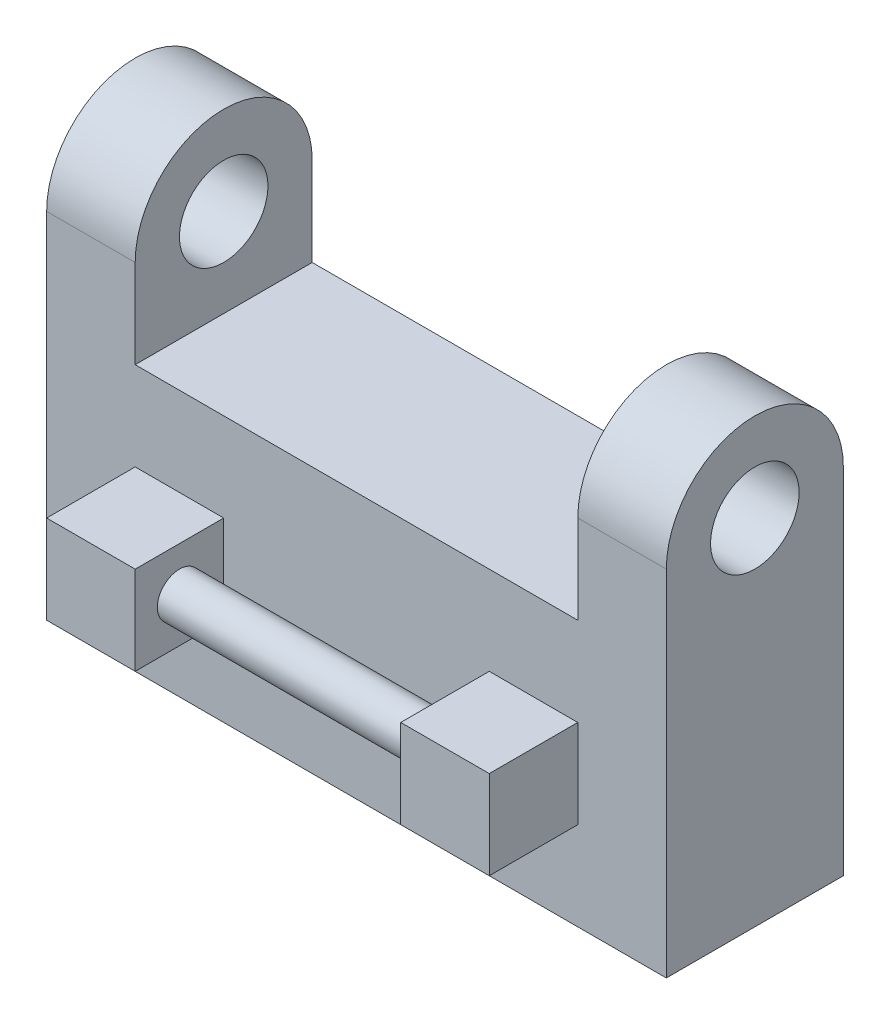
ISO-10303-21;
HEADER;
FILE_DESCRIPTION(('STEP AP214'),'2;1');
FILE_NAME('part.step','',(''),(''),'','','');
FILE_SCHEMA(('AUTOMOTIVE_DESIGN { 1 0 10303 214 1 1 1 1 }'));
ENDSEC;
DATA;
#1=APPLICATION_CONTEXT('core data for automotive mechanical design processes');
#2=APPLICATION_PROTOCOL_DEFINITION('international standard','automotive_design',2000,#1);
#3=PRODUCT_CONTEXT('',#1,'mechanical');
#4=PRODUCT('Part','Part','',(#3));
#5=PRODUCT_RELATED_PRODUCT_CATEGORY('part','',(#4));
#6=PRODUCT_DEFINITION_FORMATION('','',#4);
#7=PRODUCT_DEFINITION_CONTEXT('part definition',#1,'design');
#8=PRODUCT_DEFINITION('design','',#6,#7);
#9=PRODUCT_DEFINITION_SHAPE('','',#8);
#10=(LENGTH_UNIT() NAMED_UNIT(*) SI_UNIT(.MILLI.,.METRE.));
#11=(NAMED_UNIT(*) PLANE_ANGLE_UNIT() SI_UNIT($,.RADIAN.));
#12=(NAMED_UNIT(*) SI_UNIT($,.STERADIAN.) SOLID_ANGLE_UNIT());
#13=UNCERTAINTY_MEASURE_WITH_UNIT(LENGTH_MEASURE(1.E-05),#10,'distance_accuracy_value','');
#14=(GEOMETRIC_REPRESENTATION_CONTEXT(3) GLOBAL_UNCERTAINTY_ASSIGNED_CONTEXT((#13)) GLOBAL_UNIT_ASSIGNED_CONTEXT((#10,
#11,#12)) REPRESENTATION_CONTEXT('',''));
#15=CARTESIAN_POINT('',(0.,0.,0.));
#16=DIRECTION('',(0.,0.,1.));
#17=DIRECTION('',(1.,0.,0.));
#18=AXIS2_PLACEMENT_3D('',#15,#16,#17);
#19=CARTESIAN_POINT('',(0.,0.,20.));
#20=DIRECTION('',(0.,0.,1.));
#21=DIRECTION('',(1.,0.,0.));
#22=AXIS2_PLACEMENT_3D('',#19,#20,#21);
#23=PLANE('',#22);
#24=DIRECTION('',(0.,-1.,0.));
#25=VECTOR('',#24,1.);
#26=CARTESIAN_POINT('',(0.,30.,20.));
#27=LINE('',#26,#25);
#28=CARTESIAN_POINT('',(0.,40.,20.));
#29=VERTEX_POINT('',#28);
#30=CARTESIAN_POINT('',(0.,0.,20.));
#31=VERTEX_POINT('',#30);
#32=EDGE_CURVE('E389',#29,#31,#27,.T.);
#33=ORIENTED_EDGE('',*,*,#32,.T.);
#34=DIRECTION('',(1.,0.,0.));
#35=VECTOR('',#34,1.);
#36=CARTESIAN_POINT('',(0.,0.,20.));
#37=LINE('',#36,#35);
#38=CARTESIAN_POINT('',(70.,0.,20.));
#39=VERTEX_POINT('',#38);
#40=EDGE_CURVE('E392',#31,#39,#37,.T.);
#41=ORIENTED_EDGE('',*,*,#40,.T.);
#42=DIRECTION('',(0.,1.,0.));
#43=VECTOR('',#42,1.);
#44=CARTESIAN_POINT('',(70.,0.,20.));
#45=LINE('',#44,#43);
#46=CARTESIAN_POINT('',(70.,40.,20.));
#47=VERTEX_POINT('',#46);
#48=EDGE_CURVE('E391',#39,#47,#45,.T.);
#49=ORIENTED_EDGE('',*,*,#48,.T.);
#50=DIRECTION('',(1.,0.,0.));
#51=VECTOR('',#50,1.);
#52=CARTESIAN_POINT('',(60.,40.,20.));
#53=LINE('',#52,#51);
#54=CARTESIAN_POINT('',(60.,40.,20.));
#55=VERTEX_POINT('',#54);
#56=EDGE_CURVE('E351',#55,#47,#53,.T.);
#57=ORIENTED_EDGE('',*,*,#56,.F.);
#58=DIRECTION('',(0.,-1.,0.));
#59=VECTOR('',#58,1.);
#60=CARTESIAN_POINT('',(60.,40.,20.));
#61=LINE('',#60,#59);
#62=CARTESIAN_POINT('',(60.,30.,20.));
#63=VERTEX_POINT('',#62);
#64=EDGE_CURVE('E348',#55,#63,#61,.T.);
#65=ORIENTED_EDGE('',*,*,#64,.T.);
#66=DIRECTION('',(-1.,0.,0.));
#67=VECTOR('',#66,1.);
#68=CARTESIAN_POINT('',(70.,30.,20.));
#69=LINE('',#68,#67);
#70=CARTESIAN_POINT('',(10.,30.,20.));
#71=VERTEX_POINT('',#70);
#72=EDGE_CURVE('E398',#63,#71,#69,.T.);
#73=ORIENTED_EDGE('',*,*,#72,.T.);
#74=DIRECTION('',(0.,-1.,0.));
#75=VECTOR('',#74,1.);
#76=CARTESIAN_POINT('',(10.,40.,20.));
#77=LINE('',#76,#75);
#78=CARTESIAN_POINT('',(10.,40.,20.));
#79=VERTEX_POINT('',#78);
#80=EDGE_CURVE('E371',#79,#71,#77,.T.);
#81=ORIENTED_EDGE('',*,*,#80,.F.);
#82=DIRECTION('',(-1.,0.,0.));
#83=VECTOR('',#82,1.);
#84=CARTESIAN_POINT('',(10.,40.,20.));
#85=LINE('',#84,#83);
#86=EDGE_CURVE('E381',#79,#29,#85,.T.);
#87=ORIENTED_EDGE('',*,*,#86,.T.);
#88=EDGE_LOOP('',(#33,#41,#49,#57,#65,#73,#81,#87));
#89=FACE_BOUND('',#88,.T.);
#90=DIRECTION('',(-1.,0.,0.));
#91=VECTOR('',#90,1.);
#92=CARTESIAN_POINT('',(50.,20.,20.));
#93=LINE('',#92,#91);
#94=CARTESIAN_POINT('',(60.,20.,20.));
#95=VERTEX_POINT('',#94);
#96=CARTESIAN_POINT('',(50.,20.,20.));
#97=VERTEX_POINT('',#96);
#98=EDGE_CURVE('E316',#95,#97,#93,.T.);
#99=ORIENTED_EDGE('',*,*,#98,.F.);
#100=DIRECTION('',(0.,1.,0.));
#101=VECTOR('',#100,1.);
#102=CARTESIAN_POINT('',(60.,20.,20.));
#103=LINE('',#102,#101);
#104=CARTESIAN_POINT('',(60.,10.,20.));
#105=VERTEX_POINT('',#104);
#106=EDGE_CURVE('E304',#105,#95,#103,.T.);
#107=ORIENTED_EDGE('',*,*,#106,.F.);
#108=DIRECTION('',(1.,0.,0.));
#109=VECTOR('',#108,1.);
#110=CARTESIAN_POINT('',(50.,10.,20.));
#111=LINE('',#110,#109);
#112=CARTESIAN_POINT('',(50.,10.,20.));
#113=VERTEX_POINT('',#112);
#114=EDGE_CURVE('E309',#113,#105,#111,.T.);
#115=ORIENTED_EDGE('',*,*,#114,.F.);
#116=DIRECTION('',(0.,-1.,0.));
#117=VECTOR('',#116,1.);
#118=CARTESIAN_POINT('',(50.,20.,20.));
#119=LINE('',#118,#117);
#120=EDGE_CURVE('E322',#97,#113,#119,.T.);
#121=ORIENTED_EDGE('',*,*,#120,.F.);
#122=EDGE_LOOP('',(#99,#107,#115,#121));
#123=FACE_BOUND('',#122,.T.);
#124=DIRECTION('',(1.,0.,0.));
#125=VECTOR('',#124,1.);
#126=CARTESIAN_POINT('',(10.,10.,20.));
#127=LINE('',#126,#125);
#128=CARTESIAN_POINT('',(10.,10.,20.));
#129=VERTEX_POINT('',#128);
#130=CARTESIAN_POINT('',(20.,10.,20.));
#131=VERTEX_POINT('',#130);
#132=EDGE_CURVE('E287',#129,#131,#127,.T.);
#133=ORIENTED_EDGE('',*,*,#132,.F.);
#134=DIRECTION('',(0.,-1.,0.));
#135=VECTOR('',#134,1.);
#136=CARTESIAN_POINT('',(9.99999999999999,20.,20.));
#137=LINE('',#136,#135);
#138=CARTESIAN_POINT('',(9.99999999999999,20.,20.));
#139=VERTEX_POINT('',#138);
#140=EDGE_CURVE('E277',#139,#129,#137,.T.);
#141=ORIENTED_EDGE('',*,*,#140,.F.);
#142=DIRECTION('',(-1.,0.,0.));
#143=VECTOR('',#142,1.);
#144=CARTESIAN_POINT('',(9.99999999999999,20.,20.));
#145=LINE('',#144,#143);
#146=CARTESIAN_POINT('',(20.,20.,20.));
#147=VERTEX_POINT('',#146);
#148=EDGE_CURVE('E282',#147,#139,#145,.T.);
#149=ORIENTED_EDGE('',*,*,#148,.F.);
#150=DIRECTION('',(0.,1.,0.));
#151=VECTOR('',#150,1.);
#152=CARTESIAN_POINT('',(20.,20.,20.));
#153=LINE('',#152,#151);
#154=EDGE_CURVE('E292',#131,#147,#153,.T.);
#155=ORIENTED_EDGE('',*,*,#154,.F.);
#156=EDGE_LOOP('',(#133,#141,#149,#155));
#157=FACE_BOUND('',#156,.T.);
#158=ADVANCED_FACE('F44',(#89,#123,#157),#23,.T.);
#159=CARTESIAN_POINT('',(70.,30.,20.));
#160=DIRECTION('',(0.,-1.,0.));
#161=DIRECTION('',(0.,0.,-1.));
#162=AXIS2_PLACEMENT_3D('',#159,#160,#161);
#163=PLANE('',#162);
#164=ORIENTED_EDGE('',*,*,#72,.F.);
#165=DIRECTION('',(0.,0.,-1.));
#166=VECTOR('',#165,1.);
#167=CARTESIAN_POINT('',(60.,30.,0.));
#168=LINE('',#167,#166);
#169=CARTESIAN_POINT('',(60.,30.,0.));
#170=VERTEX_POINT('',#169);
#171=EDGE_CURVE('E350',#63,#170,#168,.T.);
#172=ORIENTED_EDGE('',*,*,#171,.T.);
#173=DIRECTION('',(-1.,0.,0.));
#174=VECTOR('',#173,1.);
#175=CARTESIAN_POINT('',(70.,30.,0.));
#176=LINE('',#175,#174);
#177=CARTESIAN_POINT('',(10.,30.,0.));
#178=VERTEX_POINT('',#177);
#179=EDGE_CURVE('E395',#170,#178,#176,.T.);
#180=ORIENTED_EDGE('',*,*,#179,.T.);
#181=DIRECTION('',(0.,0.,-1.));
#182=VECTOR('',#181,1.);
#183=CARTESIAN_POINT('',(10.,30.,0.));
#184=LINE('',#183,#182);
#185=EDGE_CURVE('E372',#71,#178,#184,.T.);
#186=ORIENTED_EDGE('',*,*,#185,.F.);
#187=EDGE_LOOP('',(#164,#172,#180,#186));
#188=FACE_BOUND('',#187,.T.);
#189=ADVANCED_FACE('F432',(#188),#163,.F.);
#190=CARTESIAN_POINT('',(0.,30.,20.));
#191=DIRECTION('',(1.,0.,0.));
#192=DIRECTION('',(0.,0.,-1.));
#193=AXIS2_PLACEMENT_3D('',#190,#191,#192);
#194=PLANE('',#193);
#195=DIRECTION('',(0.,-1.,0.));
#196=VECTOR('',#195,1.);
#197=CARTESIAN_POINT('',(0.,30.,0.));
#198=LINE('',#197,#196);
#199=CARTESIAN_POINT('',(0.,40.,0.));
#200=VERTEX_POINT('',#199);
#201=CARTESIAN_POINT('',(0.,0.,0.));
#202=VERTEX_POINT('',#201);
#203=EDGE_CURVE('E390',#200,#202,#198,.T.);
#204=ORIENTED_EDGE('',*,*,#203,.T.);
#205=DIRECTION('',(0.,0.,-1.));
#206=VECTOR('',#205,1.);
#207=CARTESIAN_POINT('',(0.,0.,20.));
#208=LINE('',#207,#206);
#209=EDGE_CURVE('E409',#31,#202,#208,.T.);
#210=ORIENTED_EDGE('',*,*,#209,.F.);
#211=ORIENTED_EDGE('',*,*,#32,.F.);
#212=CARTESIAN_POINT('',(0.,40.,10.));
#213=DIRECTION('',(1.,0.,0.));
#214=DIRECTION('',(0.,0.,-1.));
#215=AXIS2_PLACEMENT_3D('',#212,#213,#214);
#216=CIRCLE('',#215,10.);
#217=EDGE_CURVE('E362',#200,#29,#216,.T.);
#218=ORIENTED_EDGE('',*,*,#217,.F.);
#219=EDGE_LOOP('',(#204,#210,#211,#218));
#220=FACE_BOUND('',#219,.T.);
#221=CARTESIAN_POINT('',(0.,40.,10.));
#222=DIRECTION('',(1.,0.,0.));
#223=DIRECTION('',(0.,0.,-1.));
#224=AXIS2_PLACEMENT_3D('',#221,#222,#223);
#225=CIRCLE('',#224,5.);
#226=CARTESIAN_POINT('',(0.,40.,5.));
#227=VERTEX_POINT('',#226);
#228=EDGE_CURVE('E363',#227,#227,#225,.T.);
#229=ORIENTED_EDGE('',*,*,#228,.T.);
#230=EDGE_LOOP('',(#229));
#231=FACE_BOUND('',#230,.T.);
#232=ADVANCED_FACE('F50',(#220,#231),#194,.F.);
#233=CARTESIAN_POINT('',(0.,0.,20.));
#234=DIRECTION('',(0.,1.,0.));
#235=DIRECTION('',(0.,0.,1.));
#236=AXIS2_PLACEMENT_3D('',#233,#234,#235);
#237=PLANE('',#236);
#238=DIRECTION('',(1.,0.,0.));
#239=VECTOR('',#238,1.);
#240=CARTESIAN_POINT('',(0.,0.,0.));
#241=LINE('',#240,#239);
#242=CARTESIAN_POINT('',(70.,0.,0.));
#243=VERTEX_POINT('',#242);
#244=EDGE_CURVE('E402',#202,#243,#241,.T.);
#245=ORIENTED_EDGE('',*,*,#244,.T.);
#246=DIRECTION('',(0.,0.,-1.));
#247=VECTOR('',#246,1.);
#248=CARTESIAN_POINT('',(70.,0.,20.));
#249=LINE('',#248,#247);
#250=EDGE_CURVE('E396',#39,#243,#249,.T.);
#251=ORIENTED_EDGE('',*,*,#250,.F.);
#252=ORIENTED_EDGE('',*,*,#40,.F.);
#253=ORIENTED_EDGE('',*,*,#209,.T.);
#254=EDGE_LOOP('',(#245,#251,#252,#253));
#255=FACE_BOUND('',#254,.T.);
#256=ADVANCED_FACE('F451',(#255),#237,.F.);
#257=CARTESIAN_POINT('',(70.,0.,20.));
#258=DIRECTION('',(-1.,0.,0.));
#259=DIRECTION('',(0.,0.,1.));
#260=AXIS2_PLACEMENT_3D('',#257,#258,#259);
#261=PLANE('',#260);
#262=DIRECTION('',(0.,1.,0.));
#263=VECTOR('',#262,1.);
#264=CARTESIAN_POINT('',(70.,0.,0.));
#265=LINE('',#264,#263);
#266=CARTESIAN_POINT('',(70.,40.,0.));
#267=VERTEX_POINT('',#266);
#268=EDGE_CURVE('E401',#243,#267,#265,.T.);
#269=ORIENTED_EDGE('',*,*,#268,.T.);
#270=CARTESIAN_POINT('',(70.,40.,10.));
#271=DIRECTION('',(1.,0.,0.));
#272=DIRECTION('',(0.,0.,-1.));
#273=AXIS2_PLACEMENT_3D('',#270,#271,#272);
#274=CIRCLE('',#273,10.);
#275=EDGE_CURVE('E336',#267,#47,#274,.T.);
#276=ORIENTED_EDGE('',*,*,#275,.T.);
#277=ORIENTED_EDGE('',*,*,#48,.F.);
#278=ORIENTED_EDGE('',*,*,#250,.T.);
#279=EDGE_LOOP('',(#269,#276,#277,#278));
#280=FACE_BOUND('',#279,.T.);
#281=CARTESIAN_POINT('',(70.,40.,10.));
#282=DIRECTION('',(1.,0.,0.));
#283=DIRECTION('',(0.,0.,-1.));
#284=AXIS2_PLACEMENT_3D('',#281,#282,#283);
#285=CIRCLE('',#284,5.);
#286=CARTESIAN_POINT('',(70.,40.,5.));
#287=VERTEX_POINT('',#286);
#288=EDGE_CURVE('E334',#287,#287,#285,.T.);
#289=ORIENTED_EDGE('',*,*,#288,.F.);
#290=EDGE_LOOP('',(#289));
#291=FACE_BOUND('',#290,.T.);
#292=ADVANCED_FACE('F448',(#280,#291),#261,.F.);
#293=CARTESIAN_POINT('',(0.,0.,0.));
#294=DIRECTION('',(0.,0.,1.));
#295=DIRECTION('',(1.,0.,0.));
#296=AXIS2_PLACEMENT_3D('',#293,#294,#295);
#297=PLANE('',#296);
#298=DIRECTION('',(-1.,0.,0.));
#299=VECTOR('',#298,1.);
#300=CARTESIAN_POINT('',(9.99999999999999,20.,0.));
#301=LINE('',#300,#299);
#302=CARTESIAN_POINT('',(20.,20.,0.));
#303=VERTEX_POINT('',#302);
#304=CARTESIAN_POINT('',(9.99999999999999,20.,0.));
#305=VERTEX_POINT('',#304);
#306=EDGE_CURVE('E238',#303,#305,#301,.T.);
#307=ORIENTED_EDGE('',*,*,#306,.T.);
#308=DIRECTION('',(0.,-1.,0.));
#309=VECTOR('',#308,1.);
#310=CARTESIAN_POINT('',(9.99999999999999,20.,0.));
#311=LINE('',#310,#309);
#312=CARTESIAN_POINT('',(10.,10.,0.));
#313=VERTEX_POINT('',#312);
#314=EDGE_CURVE('E215',#305,#313,#311,.T.);
#315=ORIENTED_EDGE('',*,*,#314,.T.);
#316=DIRECTION('',(1.,0.,0.));
#317=VECTOR('',#316,1.);
#318=CARTESIAN_POINT('',(10.,10.,0.));
#319=LINE('',#318,#317);
#320=CARTESIAN_POINT('',(20.,10.,0.));
#321=VERTEX_POINT('',#320);
#322=EDGE_CURVE('E226',#313,#321,#319,.T.);
#323=ORIENTED_EDGE('',*,*,#322,.T.);
#324=DIRECTION('',(0.,1.,0.));
#325=VECTOR('',#324,1.);
#326=CARTESIAN_POINT('',(20.,20.,0.));
#327=LINE('',#326,#325);
#328=EDGE_CURVE('E58',#321,#303,#327,.T.);
#329=ORIENTED_EDGE('',*,*,#328,.T.);
#330=EDGE_LOOP('',(#307,#315,#323,#329));
#331=FACE_BOUND('',#330,.T.);
#332=DIRECTION('',(1.,0.,0.));
#333=VECTOR('',#332,1.);
#334=CARTESIAN_POINT('',(50.,10.,0.));
#335=LINE('',#334,#333);
#336=CARTESIAN_POINT('',(50.,10.,0.));
#337=VERTEX_POINT('',#336);
#338=CARTESIAN_POINT('',(60.,10.,0.));
#339=VERTEX_POINT('',#338);
#340=EDGE_CURVE('E264',#337,#339,#335,.T.);
#341=ORIENTED_EDGE('',*,*,#340,.T.);
#342=DIRECTION('',(0.,1.,0.));
#343=VECTOR('',#342,1.);
#344=CARTESIAN_POINT('',(60.,20.,0.));
#345=LINE('',#344,#343);
#346=CARTESIAN_POINT('',(60.,20.,0.));
#347=VERTEX_POINT('',#346);
#348=EDGE_CURVE('E220',#339,#347,#345,.T.);
#349=ORIENTED_EDGE('',*,*,#348,.T.);
#350=DIRECTION('',(-1.,0.,0.));
#351=VECTOR('',#350,1.);
#352=CARTESIAN_POINT('',(50.,20.,0.));
#353=LINE('',#352,#351);
#354=CARTESIAN_POINT('',(50.,20.,0.));
#355=VERTEX_POINT('',#354);
#356=EDGE_CURVE('E252',#347,#355,#353,.T.);
#357=ORIENTED_EDGE('',*,*,#356,.T.);
#358=DIRECTION('',(0.,-1.,0.));
#359=VECTOR('',#358,1.);
#360=CARTESIAN_POINT('',(50.,20.,0.));
#361=LINE('',#360,#359);
#362=EDGE_CURVE('E69',#355,#337,#361,.T.);
#363=ORIENTED_EDGE('',*,*,#362,.T.);
#364=EDGE_LOOP('',(#341,#349,#357,#363));
#365=FACE_BOUND('',#364,.T.);
#366=ORIENTED_EDGE('',*,*,#203,.F.);
#367=DIRECTION('',(-1.,0.,0.));
#368=VECTOR('',#367,1.);
#369=CARTESIAN_POINT('',(10.,40.,0.));
#370=LINE('',#369,#368);
#371=CARTESIAN_POINT('',(10.,40.,0.));
#372=VERTEX_POINT('',#371);
#373=EDGE_CURVE('E378',#372,#200,#370,.T.);
#374=ORIENTED_EDGE('',*,*,#373,.F.);
#375=DIRECTION('',(0.,1.,0.));
#376=VECTOR('',#375,1.);
#377=CARTESIAN_POINT('',(10.,40.,0.));
#378=LINE('',#377,#376);
#379=EDGE_CURVE('E380',#178,#372,#378,.T.);
#380=ORIENTED_EDGE('',*,*,#379,.F.);
#381=ORIENTED_EDGE('',*,*,#179,.F.);
#382=DIRECTION('',(0.,1.,0.));
#383=VECTOR('',#382,1.);
#384=CARTESIAN_POINT('',(60.,40.,0.));
#385=LINE('',#384,#383);
#386=CARTESIAN_POINT('',(60.,40.,0.));
#387=VERTEX_POINT('',#386);
#388=EDGE_CURVE('E341',#170,#387,#385,.T.);
#389=ORIENTED_EDGE('',*,*,#388,.T.);
#390=DIRECTION('',(1.,0.,0.));
#391=VECTOR('',#390,1.);
#392=CARTESIAN_POINT('',(60.,40.,0.));
#393=LINE('',#392,#391);
#394=EDGE_CURVE('E356',#387,#267,#393,.T.);
#395=ORIENTED_EDGE('',*,*,#394,.T.);
#396=ORIENTED_EDGE('',*,*,#268,.F.);
#397=ORIENTED_EDGE('',*,*,#244,.F.);
#398=EDGE_LOOP('',(#366,#374,#380,#381,#389,#395,#396,#397));
#399=FACE_BOUND('',#398,.T.);
#400=ADVANCED_FACE('F450',(#331,#365,#399),#297,.F.);
#401=CARTESIAN_POINT('',(10.,40.,10.));
#402=DIRECTION('',(1.,0.,0.));
#403=DIRECTION('',(0.,0.,-1.));
#404=AXIS2_PLACEMENT_3D('',#401,#402,#403);
#405=PLANE('',#404);
#406=CARTESIAN_POINT('',(10.,40.,10.));
#407=DIRECTION('',(1.,0.,0.));
#408=DIRECTION('',(0.,0.,-1.));
#409=AXIS2_PLACEMENT_3D('',#406,#407,#408);
#410=CIRCLE('',#409,10.);
#411=EDGE_CURVE('E368',#372,#79,#410,.T.);
#412=ORIENTED_EDGE('',*,*,#411,.T.);
#413=ORIENTED_EDGE('',*,*,#80,.T.);
#414=ORIENTED_EDGE('',*,*,#185,.T.);
#415=ORIENTED_EDGE('',*,*,#379,.T.);
#416=EDGE_LOOP('',(#412,#413,#414,#415));
#417=FACE_BOUND('',#416,.T.);
#418=CARTESIAN_POINT('',(10.,40.,10.));
#419=DIRECTION('',(1.,0.,0.));
#420=DIRECTION('',(0.,0.,-1.));
#421=AXIS2_PLACEMENT_3D('',#418,#419,#420);
#422=CIRCLE('',#421,5.);
#423=CARTESIAN_POINT('',(10.,40.,5.));
#424=VERTEX_POINT('',#423);
#425=EDGE_CURVE('E365',#424,#424,#422,.T.);
#426=ORIENTED_EDGE('',*,*,#425,.F.);
#427=EDGE_LOOP('',(#426));
#428=FACE_BOUND('',#427,.T.);
#429=ADVANCED_FACE('F446',(#417,#428),#405,.T.);
#430=CARTESIAN_POINT('',(10.,40.,10.));
#431=DIRECTION('',(-1.,0.,0.));
#432=DIRECTION('',(0.,0.,1.));
#433=AXIS2_PLACEMENT_3D('',#430,#431,#432);
#434=CYLINDRICAL_SURFACE('',#433,10.);
#435=ORIENTED_EDGE('',*,*,#217,.T.);
#436=ORIENTED_EDGE('',*,*,#86,.F.);
#437=ORIENTED_EDGE('',*,*,#411,.F.);
#438=ORIENTED_EDGE('',*,*,#373,.T.);
#439=EDGE_LOOP('',(#435,#436,#437,#438));
#440=FACE_BOUND('',#439,.T.);
#441=ADVANCED_FACE('F444',(#440),#434,.T.);
#442=CARTESIAN_POINT('',(10.,40.,10.));
#443=DIRECTION('',(-1.,0.,0.));
#444=DIRECTION('',(0.,0.,1.));
#445=AXIS2_PLACEMENT_3D('',#442,#443,#444);
#446=CYLINDRICAL_SURFACE('',#445,5.);
#447=ORIENTED_EDGE('',*,*,#425,.T.);
#448=EDGE_LOOP('',(#447));
#449=FACE_BOUND('',#448,.T.);
#450=ORIENTED_EDGE('',*,*,#228,.F.);
#451=EDGE_LOOP('',(#450));
#452=FACE_BOUND('',#451,.T.);
#453=ADVANCED_FACE('F497',(#449,#452),#446,.F.);
#454=CARTESIAN_POINT('',(60.,40.,10.));
#455=DIRECTION('',(1.,0.,0.));
#456=DIRECTION('',(0.,0.,-1.));
#457=AXIS2_PLACEMENT_3D('',#454,#455,#456);
#458=CYLINDRICAL_SURFACE('',#457,10.);
#459=ORIENTED_EDGE('',*,*,#275,.F.);
#460=ORIENTED_EDGE('',*,*,#394,.F.);
#461=CARTESIAN_POINT('',(60.,40.,10.));
#462=DIRECTION('',(1.,0.,0.));
#463=DIRECTION('',(0.,0.,-1.));
#464=AXIS2_PLACEMENT_3D('',#461,#462,#463);
#465=CIRCLE('',#464,10.);
#466=EDGE_CURVE('E342',#387,#55,#465,.T.);
#467=ORIENTED_EDGE('',*,*,#466,.T.);
#468=ORIENTED_EDGE('',*,*,#56,.T.);
#469=EDGE_LOOP('',(#459,#460,#467,#468));
#470=FACE_BOUND('',#469,.T.);
#471=ADVANCED_FACE('F474',(#470),#458,.T.);
#472=CARTESIAN_POINT('',(60.,40.,10.));
#473=DIRECTION('',(-1.,0.,0.));
#474=DIRECTION('',(0.,0.,-1.));
#475=AXIS2_PLACEMENT_3D('',#472,#473,#474);
#476=PLANE('',#475);
#477=CARTESIAN_POINT('',(60.,40.,10.));
#478=DIRECTION('',(1.,0.,0.));
#479=DIRECTION('',(0.,0.,-1.));
#480=AXIS2_PLACEMENT_3D('',#477,#478,#479);
#481=CIRCLE('',#480,5.);
#482=CARTESIAN_POINT('',(60.,40.,5.));
#483=VERTEX_POINT('',#482);
#484=EDGE_CURVE('E332',#483,#483,#481,.T.);
#485=ORIENTED_EDGE('',*,*,#484,.T.);
#486=EDGE_LOOP('',(#485));
#487=FACE_BOUND('',#486,.T.);
#488=ORIENTED_EDGE('',*,*,#466,.F.);
#489=ORIENTED_EDGE('',*,*,#388,.F.);
#490=ORIENTED_EDGE('',*,*,#171,.F.);
#491=ORIENTED_EDGE('',*,*,#64,.F.);
#492=EDGE_LOOP('',(#488,#489,#490,#491));
#493=FACE_BOUND('',#492,.T.);
#494=ADVANCED_FACE('F487',(#487,#493),#476,.T.);
#495=CARTESIAN_POINT('',(60.,40.,10.));
#496=DIRECTION('',(1.,0.,0.));
#497=DIRECTION('',(0.,0.,-1.));
#498=AXIS2_PLACEMENT_3D('',#495,#496,#497);
#499=CYLINDRICAL_SURFACE('',#498,5.);
#500=ORIENTED_EDGE('',*,*,#484,.F.);
#501=EDGE_LOOP('',(#500));
#502=FACE_BOUND('',#501,.T.);
#503=ORIENTED_EDGE('',*,*,#288,.T.);
#504=EDGE_LOOP('',(#503));
#505=FACE_BOUND('',#504,.T.);
#506=ADVANCED_FACE('F490',(#502,#505),#499,.F.);
#507=CARTESIAN_POINT('',(60.,20.,30.));
#508=DIRECTION('',(-1.,0.,0.));
#509=DIRECTION('',(0.,0.,1.));
#510=AXIS2_PLACEMENT_3D('',#507,#508,#509);
#511=PLANE('',#510);
#512=ORIENTED_EDGE('',*,*,#106,.T.);
#513=DIRECTION('',(0.,0.,-1.));
#514=VECTOR('',#513,1.);
#515=CARTESIAN_POINT('',(60.,20.,30.));
#516=LINE('',#515,#514);
#517=CARTESIAN_POINT('',(60.,20.,30.));
#518=VERTEX_POINT('',#517);
#519=EDGE_CURVE('E335',#518,#95,#516,.T.);
#520=ORIENTED_EDGE('',*,*,#519,.F.);
#521=DIRECTION('',(0.,1.,0.));
#522=VECTOR('',#521,1.);
#523=CARTESIAN_POINT('',(60.,20.,30.));
#524=LINE('',#523,#522);
#525=CARTESIAN_POINT('',(60.,10.,30.));
#526=VERTEX_POINT('',#525);
#527=EDGE_CURVE('E306',#526,#518,#524,.T.);
#528=ORIENTED_EDGE('',*,*,#527,.F.);
#529=DIRECTION('',(0.,0.,-1.));
#530=VECTOR('',#529,1.);
#531=CARTESIAN_POINT('',(60.,10.,30.));
#532=LINE('',#531,#530);
#533=EDGE_CURVE('E317',#526,#105,#532,.T.);
#534=ORIENTED_EDGE('',*,*,#533,.T.);
#535=EDGE_LOOP('',(#512,#520,#528,#534));
#536=FACE_BOUND('',#535,.T.);
#537=ADVANCED_FACE('F496',(#536),#511,.F.);
#538=CARTESIAN_POINT('',(50.,20.,30.));
#539=DIRECTION('',(0.,-1.,0.));
#540=DIRECTION('',(0.,0.,-1.));
#541=AXIS2_PLACEMENT_3D('',#538,#539,#540);
#542=PLANE('',#541);
#543=ORIENTED_EDGE('',*,*,#98,.T.);
#544=DIRECTION('',(0.,0.,-1.));
#545=VECTOR('',#544,1.);
#546=CARTESIAN_POINT('',(50.,20.,30.));
#547=LINE('',#546,#545);
#548=CARTESIAN_POINT('',(50.,20.,30.));
#549=VERTEX_POINT('',#548);
#550=EDGE_CURVE('E326',#549,#97,#547,.T.);
#551=ORIENTED_EDGE('',*,*,#550,.F.);
#552=DIRECTION('',(-1.,0.,0.));
#553=VECTOR('',#552,1.);
#554=CARTESIAN_POINT('',(50.,20.,30.));
#555=LINE('',#554,#553);
#556=EDGE_CURVE('E307',#518,#549,#555,.T.);
#557=ORIENTED_EDGE('',*,*,#556,.F.);
#558=ORIENTED_EDGE('',*,*,#519,.T.);
#559=EDGE_LOOP('',(#543,#551,#557,#558));
#560=FACE_BOUND('',#559,.T.);
#561=ADVANCED_FACE('F538',(#560),#542,.F.);
#562=CARTESIAN_POINT('',(50.,20.,30.));
#563=DIRECTION('',(1.,0.,0.));
#564=DIRECTION('',(0.,0.,-1.));
#565=AXIS2_PLACEMENT_3D('',#562,#563,#564);
#566=PLANE('',#565);
#567=CARTESIAN_POINT('',(50.,15.,25.));
#568=DIRECTION('',(1.,0.,0.));
#569=DIRECTION('',(0.,0.,-1.));
#570=AXIS2_PLACEMENT_3D('',#567,#568,#569);
#571=CIRCLE('',#570,2.5);
#572=CARTESIAN_POINT('',(50.,15.,22.5));
#573=VERTEX_POINT('',#572);
#574=EDGE_CURVE('E411',#573,#573,#571,.F.);
#575=ORIENTED_EDGE('',*,*,#574,.F.);
#576=EDGE_LOOP('',(#575));
#577=FACE_BOUND('',#576,.T.);
#578=ORIENTED_EDGE('',*,*,#120,.T.);
#579=DIRECTION('',(0.,0.,-1.));
#580=VECTOR('',#579,1.);
#581=CARTESIAN_POINT('',(50.,10.,30.));
#582=LINE('',#581,#580);
#583=CARTESIAN_POINT('',(50.,10.,30.));
#584=VERTEX_POINT('',#583);
#585=EDGE_CURVE('E330',#584,#113,#582,.T.);
#586=ORIENTED_EDGE('',*,*,#585,.F.);
#587=DIRECTION('',(0.,-1.,0.));
#588=VECTOR('',#587,1.);
#589=CARTESIAN_POINT('',(50.,20.,30.));
#590=LINE('',#589,#588);
#591=EDGE_CURVE('E315',#549,#584,#590,.T.);
#592=ORIENTED_EDGE('',*,*,#591,.F.);
#593=ORIENTED_EDGE('',*,*,#550,.T.);
#594=EDGE_LOOP('',(#578,#586,#592,#593));
#595=FACE_BOUND('',#594,.T.);
#596=ADVANCED_FACE('F547',(#577,#595),#566,.F.);
#597=CARTESIAN_POINT('',(50.,10.,30.));
#598=DIRECTION('',(0.,1.,0.));
#599=DIRECTION('',(-1.,0.,0.));
#600=AXIS2_PLACEMENT_3D('',#597,#598,#599);
#601=PLANE('',#600);
#602=ORIENTED_EDGE('',*,*,#114,.T.);
#603=ORIENTED_EDGE('',*,*,#533,.F.);
#604=DIRECTION('',(1.,0.,0.));
#605=VECTOR('',#604,1.);
#606=CARTESIAN_POINT('',(50.,10.,30.));
#607=LINE('',#606,#605);
#608=EDGE_CURVE('E313',#584,#526,#607,.T.);
#609=ORIENTED_EDGE('',*,*,#608,.F.);
#610=ORIENTED_EDGE('',*,*,#585,.T.);
#611=EDGE_LOOP('',(#602,#603,#609,#610));
#612=FACE_BOUND('',#611,.T.);
#613=ADVANCED_FACE('F561',(#612),#601,.F.);
#614=CARTESIAN_POINT('',(0.,0.,30.));
#615=DIRECTION('',(0.,0.,1.));
#616=DIRECTION('',(1.,0.,0.));
#617=AXIS2_PLACEMENT_3D('',#614,#615,#616);
#618=PLANE('',#617);
#619=ORIENTED_EDGE('',*,*,#527,.T.);
#620=ORIENTED_EDGE('',*,*,#556,.T.);
#621=ORIENTED_EDGE('',*,*,#591,.T.);
#622=ORIENTED_EDGE('',*,*,#608,.T.);
#623=EDGE_LOOP('',(#619,#620,#621,#622));
#624=FACE_BOUND('',#623,.T.);
#625=ADVANCED_FACE('F569',(#624),#618,.T.);
#626=CARTESIAN_POINT('',(9.99999999999999,20.,30.));
#627=DIRECTION('',(1.,0.,0.));
#628=DIRECTION('',(0.,1.,0.));
#629=AXIS2_PLACEMENT_3D('',#626,#627,#628);
#630=PLANE('',#629);
#631=ORIENTED_EDGE('',*,*,#140,.T.);
#632=DIRECTION('',(0.,0.,-1.));
#633=VECTOR('',#632,1.);
#634=CARTESIAN_POINT('',(10.,10.,30.));
#635=LINE('',#634,#633);
#636=CARTESIAN_POINT('',(10.,10.,30.));
#637=VERTEX_POINT('',#636);
#638=EDGE_CURVE('E303',#637,#129,#635,.T.);
#639=ORIENTED_EDGE('',*,*,#638,.F.);
#640=DIRECTION('',(0.,-1.,0.));
#641=VECTOR('',#640,1.);
#642=CARTESIAN_POINT('',(9.99999999999999,20.,30.));
#643=LINE('',#642,#641);
#644=CARTESIAN_POINT('',(9.99999999999999,20.,30.));
#645=VERTEX_POINT('',#644);
#646=EDGE_CURVE('E280',#645,#637,#643,.T.);
#647=ORIENTED_EDGE('',*,*,#646,.F.);
#648=DIRECTION('',(0.,0.,-1.));
#649=VECTOR('',#648,1.);
#650=CARTESIAN_POINT('',(9.99999999999999,20.,30.));
#651=LINE('',#650,#649);
#652=EDGE_CURVE('E290',#645,#139,#651,.T.);
#653=ORIENTED_EDGE('',*,*,#652,.T.);
#654=EDGE_LOOP('',(#631,#639,#647,#653));
#655=FACE_BOUND('',#654,.T.);
#656=ADVANCED_FACE('F572',(#655),#630,.F.);
#657=CARTESIAN_POINT('',(10.,10.,30.));
#658=DIRECTION('',(0.,1.,0.));
#659=DIRECTION('',(0.,0.,1.));
#660=AXIS2_PLACEMENT_3D('',#657,#658,#659);
#661=PLANE('',#660);
#662=ORIENTED_EDGE('',*,*,#132,.T.);
#663=DIRECTION('',(0.,0.,-1.));
#664=VECTOR('',#663,1.);
#665=CARTESIAN_POINT('',(20.,10.,30.));
#666=LINE('',#665,#664);
#667=CARTESIAN_POINT('',(20.,10.,30.));
#668=VERTEX_POINT('',#667);
#669=EDGE_CURVE('E297',#668,#131,#666,.T.);
#670=ORIENTED_EDGE('',*,*,#669,.F.);
#671=DIRECTION('',(1.,0.,0.));
#672=VECTOR('',#671,1.);
#673=CARTESIAN_POINT('',(10.,10.,30.));
#674=LINE('',#673,#672);
#675=EDGE_CURVE('E278',#637,#668,#674,.T.);
#676=ORIENTED_EDGE('',*,*,#675,.F.);
#677=ORIENTED_EDGE('',*,*,#638,.T.);
#678=EDGE_LOOP('',(#662,#670,#676,#677));
#679=FACE_BOUND('',#678,.T.);
#680=ADVANCED_FACE('F584',(#679),#661,.F.);
#681=CARTESIAN_POINT('',(20.,20.,30.));
#682=DIRECTION('',(-1.,0.,0.));
#683=DIRECTION('',(0.,0.,1.));
#684=AXIS2_PLACEMENT_3D('',#681,#682,#683);
#685=PLANE('',#684);
#686=CARTESIAN_POINT('',(20.,15.,25.));
#687=DIRECTION('',(-1.,0.,0.));
#688=DIRECTION('',(0.,0.,1.));
#689=AXIS2_PLACEMENT_3D('',#686,#687,#688);
#690=CIRCLE('',#689,2.5);
#691=CARTESIAN_POINT('',(20.,15.,27.5));
#692=VERTEX_POINT('',#691);
#693=EDGE_CURVE('E412',#692,#692,#690,.F.);
#694=ORIENTED_EDGE('',*,*,#693,.F.);
#695=EDGE_LOOP('',(#694));
#696=FACE_BOUND('',#695,.T.);
#697=ORIENTED_EDGE('',*,*,#154,.T.);
#698=DIRECTION('',(0.,0.,-1.));
#699=VECTOR('',#698,1.);
#700=CARTESIAN_POINT('',(20.,20.,30.));
#701=LINE('',#700,#699);
#702=CARTESIAN_POINT('',(20.,20.,30.));
#703=VERTEX_POINT('',#702);
#704=EDGE_CURVE('E296',#703,#147,#701,.T.);
#705=ORIENTED_EDGE('',*,*,#704,.F.);
#706=DIRECTION('',(0.,1.,0.));
#707=VECTOR('',#706,1.);
#708=CARTESIAN_POINT('',(20.,20.,30.));
#709=LINE('',#708,#707);
#710=EDGE_CURVE('E284',#668,#703,#709,.T.);
#711=ORIENTED_EDGE('',*,*,#710,.F.);
#712=ORIENTED_EDGE('',*,*,#669,.T.);
#713=EDGE_LOOP('',(#697,#705,#711,#712));
#714=FACE_BOUND('',#713,.T.);
#715=ADVANCED_FACE('F593',(#696,#714),#685,.F.);
#716=CARTESIAN_POINT('',(9.99999999999999,20.,30.));
#717=DIRECTION('',(0.,-1.,0.));
#718=DIRECTION('',(0.,0.,-1.));
#719=AXIS2_PLACEMENT_3D('',#716,#717,#718);
#720=PLANE('',#719);
#721=ORIENTED_EDGE('',*,*,#148,.T.);
#722=ORIENTED_EDGE('',*,*,#652,.F.);
#723=DIRECTION('',(-1.,0.,0.));
#724=VECTOR('',#723,1.);
#725=CARTESIAN_POINT('',(9.99999999999999,20.,30.));
#726=LINE('',#725,#724);
#727=EDGE_CURVE('E283',#703,#645,#726,.T.);
#728=ORIENTED_EDGE('',*,*,#727,.F.);
#729=ORIENTED_EDGE('',*,*,#704,.T.);
#730=EDGE_LOOP('',(#721,#722,#728,#729));
#731=FACE_BOUND('',#730,.T.);
#732=ADVANCED_FACE('F594',(#731),#720,.F.);
#733=CARTESIAN_POINT('',(0.,0.,30.));
#734=DIRECTION('',(0.,0.,1.));
#735=DIRECTION('',(1.,0.,0.));
#736=AXIS2_PLACEMENT_3D('',#733,#734,#735);
#737=PLANE('',#736);
#738=ORIENTED_EDGE('',*,*,#646,.T.);
#739=ORIENTED_EDGE('',*,*,#675,.T.);
#740=ORIENTED_EDGE('',*,*,#710,.T.);
#741=ORIENTED_EDGE('',*,*,#727,.T.);
#742=EDGE_LOOP('',(#738,#739,#740,#741));
#743=FACE_BOUND('',#742,.T.);
#744=ADVANCED_FACE('F601',(#743),#737,.T.);
#745=CARTESIAN_POINT('',(50.,15.,25.));
#746=DIRECTION('',(-1.,0.,0.));
#747=DIRECTION('',(0.,0.,1.));
#748=AXIS2_PLACEMENT_3D('',#745,#746,#747);
#749=CYLINDRICAL_SURFACE('',#748,2.5);
#750=ORIENTED_EDGE('',*,*,#574,.T.);
#751=EDGE_LOOP('',(#750));
#752=FACE_BOUND('',#751,.T.);
#753=ORIENTED_EDGE('',*,*,#693,.T.);
#754=EDGE_LOOP('',(#753));
#755=FACE_BOUND('',#754,.T.);
#756=ADVANCED_FACE('F611',(#752,#755),#749,.T.);
#757=CARTESIAN_POINT('',(60.,20.,-10.));
#758=DIRECTION('',(1.,0.,0.));
#759=DIRECTION('',(0.,0.,-1.));
#760=AXIS2_PLACEMENT_3D('',#757,#758,#759);
#761=PLANE('',#760);
#762=ORIENTED_EDGE('',*,*,#348,.F.);
#763=DIRECTION('',(0.,0.,1.));
#764=VECTOR('',#763,1.);
#765=CARTESIAN_POINT('',(60.,10.,-10.));
#766=LINE('',#765,#764);
#767=CARTESIAN_POINT('',(60.,10.,-10.));
#768=VERTEX_POINT('',#767);
#769=EDGE_CURVE('E274',#768,#339,#766,.T.);
#770=ORIENTED_EDGE('',*,*,#769,.F.);
#771=DIRECTION('',(0.,1.,0.));
#772=VECTOR('',#771,1.);
#773=CARTESIAN_POINT('',(60.,20.,-10.));
#774=LINE('',#773,#772);
#775=CARTESIAN_POINT('',(60.,20.,-10.));
#776=VERTEX_POINT('',#775);
#777=EDGE_CURVE('E250',#768,#776,#774,.T.);
#778=ORIENTED_EDGE('',*,*,#777,.T.);
#779=DIRECTION('',(0.,0.,1.));
#780=VECTOR('',#779,1.);
#781=CARTESIAN_POINT('',(60.,20.,-10.));
#782=LINE('',#781,#780);
#783=EDGE_CURVE('E258',#776,#347,#782,.T.);
#784=ORIENTED_EDGE('',*,*,#783,.T.);
#785=EDGE_LOOP('',(#762,#770,#778,#784));
#786=FACE_BOUND('',#785,.T.);
#787=ADVANCED_FACE('F619',(#786),#761,.T.);
#788=CARTESIAN_POINT('',(50.,10.,-10.));
#789=DIRECTION('',(0.,-1.,0.));
#790=DIRECTION('',(1.,0.,0.));
#791=AXIS2_PLACEMENT_3D('',#788,#789,#790);
#792=PLANE('',#791);
#793=ORIENTED_EDGE('',*,*,#340,.F.);
#794=DIRECTION('',(0.,0.,1.));
#795=VECTOR('',#794,1.);
#796=CARTESIAN_POINT('',(50.,10.,-10.));
#797=LINE('',#796,#795);
#798=CARTESIAN_POINT('',(50.,10.,-10.));
#799=VERTEX_POINT('',#798);
#800=EDGE_CURVE('E275',#799,#337,#797,.T.);
#801=ORIENTED_EDGE('',*,*,#800,.F.);
#802=DIRECTION('',(1.,0.,0.));
#803=VECTOR('',#802,1.);
#804=CARTESIAN_POINT('',(50.,10.,-10.));
#805=LINE('',#804,#803);
#806=EDGE_CURVE('E249',#799,#768,#805,.T.);
#807=ORIENTED_EDGE('',*,*,#806,.T.);
#808=ORIENTED_EDGE('',*,*,#769,.T.);
#809=EDGE_LOOP('',(#793,#801,#807,#808));
#810=FACE_BOUND('',#809,.T.);
#811=ADVANCED_FACE('F624',(#810),#792,.T.);
#812=CARTESIAN_POINT('',(50.,20.,-10.));
#813=DIRECTION('',(-1.,0.,0.));
#814=DIRECTION('',(0.,0.,1.));
#815=AXIS2_PLACEMENT_3D('',#812,#813,#814);
#816=PLANE('',#815);
#817=CARTESIAN_POINT('',(50.,15.,-5.));
#818=DIRECTION('',(-1.,0.,0.));
#819=DIRECTION('',(0.,0.,1.));
#820=AXIS2_PLACEMENT_3D('',#817,#818,#819);
#821=CIRCLE('',#820,2.5);
#822=CARTESIAN_POINT('',(50.,15.,-2.5));
#823=VERTEX_POINT('',#822);
#824=EDGE_CURVE('E11',#823,#823,#821,.T.);
#825=ORIENTED_EDGE('',*,*,#824,.F.);
#826=EDGE_LOOP('',(#825));
#827=FACE_BOUND('',#826,.T.);
#828=ORIENTED_EDGE('',*,*,#362,.F.);
#829=DIRECTION('',(0.,0.,1.));
#830=VECTOR('',#829,1.);
#831=CARTESIAN_POINT('',(50.,20.,-10.));
#832=LINE('',#831,#830);
#833=CARTESIAN_POINT('',(50.,20.,-10.));
#834=VERTEX_POINT('',#833);
#835=EDGE_CURVE('E267',#834,#355,#832,.T.);
#836=ORIENTED_EDGE('',*,*,#835,.F.);
#837=DIRECTION('',(0.,-1.,0.));
#838=VECTOR('',#837,1.);
#839=CARTESIAN_POINT('',(50.,20.,-10.));
#840=LINE('',#839,#838);
#841=EDGE_CURVE('E251',#834,#799,#840,.T.);
#842=ORIENTED_EDGE('',*,*,#841,.T.);
#843=ORIENTED_EDGE('',*,*,#800,.T.);
#844=EDGE_LOOP('',(#828,#836,#842,#843));
#845=FACE_BOUND('',#844,.T.);
#846=ADVANCED_FACE('F635',(#827,#845),#816,.T.);
#847=CARTESIAN_POINT('',(50.,20.,-10.));
#848=DIRECTION('',(0.,1.,0.));
#849=DIRECTION('',(0.,0.,1.));
#850=AXIS2_PLACEMENT_3D('',#847,#848,#849);
#851=PLANE('',#850);
#852=ORIENTED_EDGE('',*,*,#356,.F.);
#853=ORIENTED_EDGE('',*,*,#783,.F.);
#854=DIRECTION('',(-1.,0.,0.));
#855=VECTOR('',#854,1.);
#856=CARTESIAN_POINT('',(50.,20.,-10.));
#857=LINE('',#856,#855);
#858=EDGE_CURVE('E260',#776,#834,#857,.T.);
#859=ORIENTED_EDGE('',*,*,#858,.T.);
#860=ORIENTED_EDGE('',*,*,#835,.T.);
#861=EDGE_LOOP('',(#852,#853,#859,#860));
#862=FACE_BOUND('',#861,.T.);
#863=ADVANCED_FACE('F636',(#862),#851,.T.);
#864=CARTESIAN_POINT('',(0.,0.,-10.));
#865=DIRECTION('',(0.,0.,-1.));
#866=DIRECTION('',(1.,0.,0.));
#867=AXIS2_PLACEMENT_3D('',#864,#865,#866);
#868=PLANE('',#867);
#869=ORIENTED_EDGE('',*,*,#777,.F.);
#870=ORIENTED_EDGE('',*,*,#806,.F.);
#871=ORIENTED_EDGE('',*,*,#841,.F.);
#872=ORIENTED_EDGE('',*,*,#858,.F.);
#873=EDGE_LOOP('',(#869,#870,#871,#872));
#874=FACE_BOUND('',#873,.T.);
#875=ADVANCED_FACE('F650',(#874),#868,.T.);
#876=CARTESIAN_POINT('',(9.99999999999999,20.,-10.));
#877=DIRECTION('',(-1.,0.,0.));
#878=DIRECTION('',(0.,-1.,0.));
#879=AXIS2_PLACEMENT_3D('',#876,#877,#878);
#880=PLANE('',#879);
#881=ORIENTED_EDGE('',*,*,#314,.F.);
#882=DIRECTION('',(0.,0.,1.));
#883=VECTOR('',#882,1.);
#884=CARTESIAN_POINT('',(9.99999999999999,20.,-10.));
#885=LINE('',#884,#883);
#886=CARTESIAN_POINT('',(9.99999999999999,20.,-10.));
#887=VERTEX_POINT('',#886);
#888=EDGE_CURVE('E207',#887,#305,#885,.T.);
#889=ORIENTED_EDGE('',*,*,#888,.F.);
#890=DIRECTION('',(0.,-1.,0.));
#891=VECTOR('',#890,1.);
#892=CARTESIAN_POINT('',(9.99999999999999,20.,-10.));
#893=LINE('',#892,#891);
#894=CARTESIAN_POINT('',(10.,10.,-10.));
#895=VERTEX_POINT('',#894);
#896=EDGE_CURVE('E209',#887,#895,#893,.T.);
#897=ORIENTED_EDGE('',*,*,#896,.T.);
#898=DIRECTION('',(0.,0.,1.));
#899=VECTOR('',#898,1.);
#900=CARTESIAN_POINT('',(10.,10.,-10.));
#901=LINE('',#900,#899);
#902=EDGE_CURVE('E236',#895,#313,#901,.T.);
#903=ORIENTED_EDGE('',*,*,#902,.T.);
#904=EDGE_LOOP('',(#881,#889,#897,#903));
#905=FACE_BOUND('',#904,.T.);
#906=ADVANCED_FACE('F206',(#905),#880,.T.);
#907=CARTESIAN_POINT('',(9.99999999999999,20.,-10.));
#908=DIRECTION('',(0.,1.,0.));
#909=DIRECTION('',(0.,0.,1.));
#910=AXIS2_PLACEMENT_3D('',#907,#908,#909);
#911=PLANE('',#910);
#912=ORIENTED_EDGE('',*,*,#306,.F.);
#913=DIRECTION('',(0.,0.,1.));
#914=VECTOR('',#913,1.);
#915=CARTESIAN_POINT('',(20.,20.,-10.));
#916=LINE('',#915,#914);
#917=CARTESIAN_POINT('',(20.,20.,-10.));
#918=VERTEX_POINT('',#917);
#919=EDGE_CURVE('E219',#918,#303,#916,.T.);
#920=ORIENTED_EDGE('',*,*,#919,.F.);
#921=DIRECTION('',(-1.,0.,0.));
#922=VECTOR('',#921,1.);
#923=CARTESIAN_POINT('',(9.99999999999999,20.,-10.));
#924=LINE('',#923,#922);
#925=EDGE_CURVE('E224',#918,#887,#924,.T.);
#926=ORIENTED_EDGE('',*,*,#925,.T.);
#927=ORIENTED_EDGE('',*,*,#888,.T.);
#928=EDGE_LOOP('',(#912,#920,#926,#927));
#929=FACE_BOUND('',#928,.T.);
#930=ADVANCED_FACE('F229',(#929),#911,.T.);
#931=CARTESIAN_POINT('',(20.,20.,-10.));
#932=DIRECTION('',(1.,0.,0.));
#933=DIRECTION('',(0.,0.,-1.));
#934=AXIS2_PLACEMENT_3D('',#931,#932,#933);
#935=PLANE('',#934);
#936=CARTESIAN_POINT('',(20.,15.,-5.));
#937=DIRECTION('',(1.,0.,0.));
#938=DIRECTION('',(0.,0.,-1.));
#939=AXIS2_PLACEMENT_3D('',#936,#937,#938);
#940=CIRCLE('',#939,2.5);
#941=CARTESIAN_POINT('',(20.,15.,-7.5));
#942=VERTEX_POINT('',#941);
#943=EDGE_CURVE('E52',#942,#942,#940,.T.);
#944=ORIENTED_EDGE('',*,*,#943,.F.);
#945=EDGE_LOOP('',(#944));
#946=FACE_BOUND('',#945,.T.);
#947=ORIENTED_EDGE('',*,*,#328,.F.);
#948=DIRECTION('',(0.,0.,1.));
#949=VECTOR('',#948,1.);
#950=CARTESIAN_POINT('',(20.,10.,-10.));
#951=LINE('',#950,#949);
#952=CARTESIAN_POINT('',(20.,10.,-10.));
#953=VERTEX_POINT('',#952);
#954=EDGE_CURVE('E242',#953,#321,#951,.T.);
#955=ORIENTED_EDGE('',*,*,#954,.F.);
#956=DIRECTION('',(0.,1.,0.));
#957=VECTOR('',#956,1.);
#958=CARTESIAN_POINT('',(20.,20.,-10.));
#959=LINE('',#958,#957);
#960=EDGE_CURVE('E233',#953,#918,#959,.T.);
#961=ORIENTED_EDGE('',*,*,#960,.T.);
#962=ORIENTED_EDGE('',*,*,#919,.T.);
#963=EDGE_LOOP('',(#947,#955,#961,#962));
#964=FACE_BOUND('',#963,.T.);
#965=ADVANCED_FACE('F423',(#946,#964),#935,.T.);
#966=CARTESIAN_POINT('',(10.,10.,-10.));
#967=DIRECTION('',(0.,-1.,0.));
#968=DIRECTION('',(0.,0.,-1.));
#969=AXIS2_PLACEMENT_3D('',#966,#967,#968);
#970=PLANE('',#969);
#971=ORIENTED_EDGE('',*,*,#322,.F.);
#972=ORIENTED_EDGE('',*,*,#902,.F.);
#973=DIRECTION('',(1.,0.,0.));
#974=VECTOR('',#973,1.);
#975=CARTESIAN_POINT('',(10.,10.,-10.));
#976=LINE('',#975,#974);
#977=EDGE_CURVE('E227',#895,#953,#976,.T.);
#978=ORIENTED_EDGE('',*,*,#977,.T.);
#979=ORIENTED_EDGE('',*,*,#954,.T.);
#980=EDGE_LOOP('',(#971,#972,#978,#979));
#981=FACE_BOUND('',#980,.T.);
#982=ADVANCED_FACE('F421',(#981),#970,.T.);
#983=CARTESIAN_POINT('',(0.,0.,-10.));
#984=DIRECTION('',(0.,0.,-1.));
#985=DIRECTION('',(1.,0.,0.));
#986=AXIS2_PLACEMENT_3D('',#983,#984,#985);
#987=PLANE('',#986);
#988=ORIENTED_EDGE('',*,*,#896,.F.);
#989=ORIENTED_EDGE('',*,*,#925,.F.);
#990=ORIENTED_EDGE('',*,*,#960,.F.);
#991=ORIENTED_EDGE('',*,*,#977,.F.);
#992=EDGE_LOOP('',(#988,#989,#990,#991));
#993=FACE_BOUND('',#992,.T.);
#994=ADVANCED_FACE('F225',(#993),#987,.T.);
#995=CARTESIAN_POINT('',(50.,15.,-5.));
#996=DIRECTION('',(-1.,0.,0.));
#997=DIRECTION('',(0.,0.,1.));
#998=AXIS2_PLACEMENT_3D('',#995,#996,#997);
#999=CYLINDRICAL_SURFACE('',#998,2.5);
#1000=ORIENTED_EDGE('',*,*,#824,.T.);
#1001=EDGE_LOOP('',(#1000));
#1002=FACE_BOUND('',#1001,.T.);
#1003=ORIENTED_EDGE('',*,*,#943,.T.);
#1004=EDGE_LOOP('',(#1003));
#1005=FACE_BOUND('',#1004,.T.);
#1006=ADVANCED_FACE('F419',(#1002,#1005),#999,.T.);
#1007=CLOSED_SHELL('',(#158,#189,#232,#256,#292,#400,#429,#441,#453,#471,#494,#506,#537,#561,
#596,#613,#625,#656,#680,#715,#732,#744,#756,#787,#811,#846,#863,#875,#906,#930,#965,#982,#994,#1006));
#1008=MANIFOLD_SOLID_BREP('B2',#1007);
#1009=ADVANCED_BREP_SHAPE_REPRESENTATION('',(#18,#1008),#14);
#1010=SHAPE_DEFINITION_REPRESENTATION(#9,#1009);
ENDSEC;
END-ISO-10303-21;
